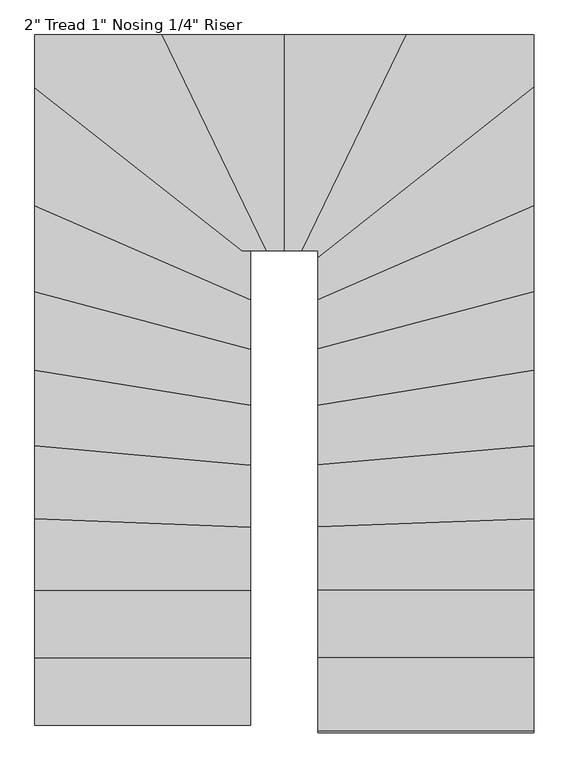
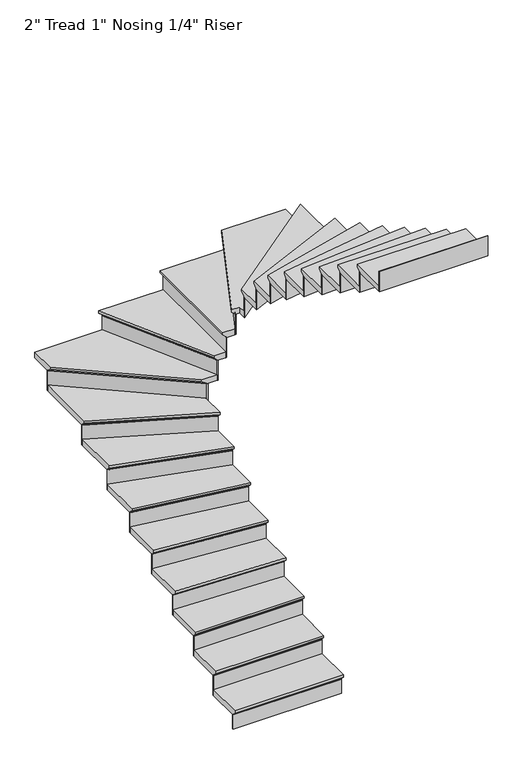
"""IFC4 building model written with IfcOpenShell, lengths in millimetres: stair flight geometry."""

from ifc_helpers import new_model, si_unit, origin, place, context, project, spatial, faceted_brep, source, transform, mapped, element, save


def stair_flight_696a7c4e(model_context):
    return source(origin(), model_context, "Body", "Brep", [
        faceted_brep([(-5047.1987704, -4554.2130548, 7470.3214286), (-5047.1987704, -4554.2130548, 7489.3714286), (-5940.8822214, -4554.2130548, 7489.3714286), (-5940.8822214, -4554.2130548, 7470.3214286), (-5047.1987704, -4528.8130548, 7444.9214286), (-5940.8822214, -4528.8130548, 7444.9214286), (-5047.1987704, -4249.4130548, 7489.3714286), (-5940.8822214, -4249.4130548, 7489.3714286), (-5940.8822214, -4528.8130548, 7438.5714286), (-5940.8822214, -4249.4130548, 7438.5714286), (-5047.1987704, -4249.4130548, 7438.5714286), (-5047.1987704, -4528.8130548, 7438.5714286)], [[[0, 1, 2, 3]], [[4, 0, 3, 5]], [[2, 1, 6, 7]], [[8, 9, 10, 11]], [[2, 7, 9, 8, 5, 3]], [[8, 11, 4, 5]], [[6, 1, 0, 4, 11, 10]], [[7, 6, 10, 9]]]),
        faceted_brep([(-5047.1987704, -4528.8130548, 7438.5714286), (-5047.1987704, -4528.8130548, 7315.2), (-5047.1987704, -4522.4630548, 7315.2), (-5047.1987704, -4522.4630548, 7438.5714286), (-5940.8822214, -4528.8130548, 7438.5714286), (-5940.8822214, -4522.4630548, 7438.5714286), (-5940.8822214, -4522.4630548, 7315.2), (-5940.8822214, -4528.8130548, 7315.2)], [[[0, 1, 2, 3]], [[4, 5, 6, 7]], [[1, 0, 4, 7]], [[2, 1, 7, 6]], [[3, 2, 6, 5]], [[0, 3, 5, 4]]]),
        faceted_brep([(-5047.1987704, -4249.4130548, 7612.7428571), (-5047.1987704, -4249.4130548, 7438.5714286), (-5047.1987704, -4243.0630548, 7438.5714286), (-5047.1987704, -4243.0630548, 7612.7428571), (-5940.8822214, -4249.4130548, 7612.7428571), (-5940.8822214, -4243.0630548, 7612.7428571), (-5940.8822214, -4243.0630548, 7438.5714286), (-5940.8822214, -4249.4130548, 7438.5714286)], [[[0, 1, 2, 3]], [[4, 5, 6, 7]], [[1, 0, 4, 7]], [[2, 1, 7, 6]], [[3, 2, 6, 5]], [[0, 3, 5, 4]]]),
        faceted_brep([(-5940.8822214, -4274.8130548, 7663.5428571), (-5047.1987704, -4274.8130548, 7663.5428571), (-5047.1987704, -3970.0130548, 7663.5428571), (-5940.8822214, -3970.0130548, 7663.5428571), (-5940.8822214, -4249.4130548, 7612.7428571), (-5940.8822214, -3970.0130548, 7612.7428571), (-5047.1987704, -3970.0130548, 7612.7428571), (-5047.1987704, -4249.4130548, 7612.7428571), (-5940.8822214, -4249.4130548, 7619.0928571), (-5940.8822214, -4274.8130548, 7644.4928571), (-5047.1987704, -4249.4130548, 7619.0928571), (-5047.1987704, -4274.8130548, 7644.4928571)], [[[0, 1, 2, 3]], [[4, 5, 6, 7]], [[0, 3, 5, 4, 8, 9]], [[4, 7, 10, 8]], [[2, 1, 11, 10, 7, 6]], [[3, 2, 6, 5]], [[11, 1, 0, 9]], [[10, 11, 9, 8]]]),
        faceted_brep([(-5047.1987704, -3970.0130548, 7786.9142857), (-5047.1987704, -3970.0130548, 7612.7428571), (-5047.1987704, -3963.6630548, 7612.7428571), (-5047.1987704, -3963.6630548, 7786.9142857), (-5940.8822214, -3970.0130548, 7786.9142857), (-5940.8822214, -3963.6630548, 7786.9142857), (-5940.8822214, -3963.6630548, 7612.7428571), (-5940.8822214, -3970.0130548, 7612.7428571)], [[[0, 1, 2, 3]], [[4, 5, 6, 7]], [[1, 0, 4, 7]], [[2, 1, 7, 6]], [[3, 2, 6, 5]], [[0, 3, 5, 4]]]),
        faceted_brep([(-5940.8822214, -3995.4130548, 7837.7142857), (-5047.1987704, -3995.4130548, 7837.7142857), (-5047.1987704, -3707.9036879, 7837.7142857), (-5940.8822214, -3673.2843203, 7837.7142857), (-5940.8822214, -3970.0130548, 7786.9142857), (-5940.8822214, -3673.2843203, 7786.9142857), (-5047.1987704, -3707.9036879, 7786.9142857), (-5047.1987704, -3970.0130548, 7786.9142857), (-5940.8822214, -3970.0130548, 7793.2642857), (-5940.8822214, -3995.4130548, 7818.6642857), (-5047.1987704, -3970.0130548, 7793.2642857), (-5047.1987704, -3995.4130548, 7818.6642857)], [[[0, 1, 2, 3]], [[4, 5, 6, 7]], [[0, 3, 5, 4, 8, 9]], [[4, 7, 10, 8]], [[2, 1, 11, 10, 7, 6]], [[3, 2, 6, 5]], [[11, 1, 0, 9]], [[10, 11, 9, 8]]]),
        faceted_brep([(-5047.1987704, -3707.9036879, 7961.0857143), (-5047.1987704, -3707.9036879, 7786.9142857), (-5047.1987704, -3701.5489252, 7786.9142857), (-5047.1987704, -3701.5489252, 7961.0857143), (-5940.8822214, -3673.2843203, 7961.0857143), (-5940.8822214, -3666.9295576, 7961.0857143), (-5940.8822214, -3666.9295576, 7786.9142857), (-5940.8822214, -3673.2843203, 7786.9142857)], [[[0, 1, 2, 3]], [[4, 5, 6, 7]], [[1, 0, 4, 7]], [[2, 1, 7, 6]], [[3, 2, 6, 5]], [[0, 3, 5, 4]]]),
        faceted_brep([(-5940.8822214, -3698.703371, 8011.8857143), (-5047.1987704, -3733.3227386, 8011.8857143), (-5047.1987704, -3451.3234819, 8011.8857143), (-5940.8822214, -3370.89733, 8011.8857143), (-5940.8822214, -3673.2843203, 7961.0857143), (-5940.8822214, -3370.89733, 7961.0857143), (-5047.1987704, -3451.3234819, 7961.0857143), (-5047.1987704, -3707.9036879, 7961.0857143), (-5940.8822214, -3673.2843203, 7967.4357143), (-5940.8822214, -3698.703371, 7992.8357143), (-5047.1987704, -3707.9036879, 7967.4357143), (-5047.1987704, -3733.3227386, 7992.8357143)], [[[0, 1, 2, 3]], [[4, 5, 6, 7]], [[0, 3, 5, 4, 8, 9]], [[4, 7, 10, 8]], [[2, 1, 11, 10, 7, 6]], [[3, 2, 6, 5]], [[11, 1, 0, 9]], [[10, 11, 9, 8]]]),
        faceted_brep([(-5047.1987704, -3451.3234819, 8135.2571429), (-5047.1987704, -3451.3234819, 7961.0857143), (-5047.1987704, -3444.9478197, 7961.0857143), (-5047.1987704, -3444.9478197, 8135.2571429), (-5940.8822214, -3370.89733, 8135.2571429), (-5940.8822214, -3364.5216678, 8135.2571429), (-5940.8822214, -3364.5216678, 7961.0857143), (-5940.8822214, -3370.89733, 7961.0857143)], [[[0, 1, 2, 3]], [[4, 5, 6, 7]], [[1, 0, 4, 7]], [[2, 1, 7, 6]], [[3, 2, 6, 5]], [[0, 3, 5, 4]]]),
        faceted_brep([(-5940.8822214, -3396.3999789, 8186.0571429), (-5047.1987704, -3476.8261308, 8186.0571429), (-5047.1987704, -3203.4301079, 8186.0571429), (-5940.8822214, -3059.5417727, 8186.0571429), (-5940.8822214, -3370.89733, 8135.2571429), (-5940.8822214, -3059.5417727, 8135.2571429), (-5047.1987704, -3203.4301079, 8135.2571429), (-5047.1987704, -3451.3234819, 8135.2571429), (-5940.8822214, -3370.89733, 8141.6071429), (-5940.8822214, -3396.3999789, 8167.0071429), (-5047.1987704, -3451.3234819, 8141.6071429), (-5047.1987704, -3476.8261308, 8167.0071429)], [[[0, 1, 2, 3]], [[4, 5, 6, 7]], [[0, 3, 5, 4, 8, 9]], [[4, 7, 10, 8]], [[2, 1, 11, 10, 7, 6]], [[3, 2, 6, 5]], [[11, 1, 0, 9]], [[10, 11, 9, 8]]]),
        faceted_brep([(-5047.1987704, -3203.4301079, 8309.4285714), (-5047.1987704, -3203.4301079, 8135.2571429), (-5047.1987704, -3196.9983292, 8135.2571429), (-5047.1987704, -3196.9983292, 8309.4285714), (-5940.8822214, -3059.5417727, 8309.4285714), (-5940.8822214, -3053.109994, 8309.4285714), (-5940.8822214, -3053.109994, 8135.2571429), (-5940.8822214, -3059.5417727, 8135.2571429)], [[[0, 1, 2, 3]], [[4, 5, 6, 7]], [[1, 0, 4, 7]], [[2, 1, 7, 6]], [[3, 2, 6, 5]], [[0, 3, 5, 4]]]),
        faceted_brep([(-5940.8822214, -3085.2688872, 8360.2285714), (-5047.1987704, -3229.1572224, 8360.2285714), (-5047.1987704, -2970.3553609, 8360.2285714), (-5940.8822214, -2732.7052783, 8360.2285714), (-5940.8822214, -3059.5417727, 8309.4285714), (-5940.8822214, -2732.7052783, 8309.4285714), (-5047.1987704, -2970.3553609, 8309.4285714), (-5047.1987704, -3203.4301079, 8309.4285714), (-5940.8822214, -3059.5417727, 8315.7785714), (-5940.8822214, -3085.2688872, 8341.1785714), (-5047.1987704, -3203.4301079, 8315.7785714), (-5047.1987704, -3229.1572224, 8341.1785714)], [[[0, 1, 2, 3]], [[4, 5, 6, 7]], [[0, 3, 5, 4, 8, 9]], [[4, 7, 10, 8]], [[2, 1, 11, 10, 7, 6]], [[3, 2, 6, 5]], [[11, 1, 0, 9]], [[10, 11, 9, 8]]]),
        faceted_brep([(-5047.1987704, -2970.3553609, 8483.6), (-5047.1987704, -2970.3553609, 8309.4285714), (-5047.1987704, -2963.7846771, 8309.4285714), (-5047.1987704, -2963.7846771, 8483.6), (-5940.8822214, -2732.7052783, 8483.6), (-5940.8822214, -2726.1345945, 8483.6), (-5940.8822214, -2726.1345945, 8309.4285714), (-5940.8822214, -2732.7052783, 8309.4285714)], [[[0, 1, 2, 3]], [[4, 5, 6, 7]], [[1, 0, 4, 7]], [[2, 1, 7, 6]], [[3, 2, 6, 5]], [[0, 3, 5, 4]]]),
        faceted_brep([(-5940.8822214, -2758.9880136, 8534.4), (-5047.1987704, -2996.6380961, 8534.4), (-5047.1987704, -2765.8050203, 8534.4), (-5940.8822214, -2375.5896532, 8534.4), (-5940.8822214, -2732.7052783, 8483.6), (-5940.8822214, -2375.5896532, 8483.6), (-5047.1987704, -2765.8050203, 8483.6), (-5047.1987704, -2970.3553609, 8483.6), (-5940.8822214, -2732.7052783, 8489.95), (-5940.8822214, -2758.9880136, 8515.35), (-5047.1987704, -2970.3553609, 8489.95), (-5047.1987704, -2996.6380961, 8515.35)], [[[0, 1, 2, 3]], [[4, 5, 6, 7]], [[0, 3, 5, 4, 8, 9]], [[4, 7, 10, 8]], [[2, 1, 11, 10, 7, 6]], [[3, 2, 6, 5]], [[11, 1, 0, 9]], [[10, 11, 9, 8]]]),
        faceted_brep([(-5047.1987704, -2765.8050203, 8657.7714286), (-5047.1987704, -2765.8050203, 8483.6), (-5047.1987704, -2758.8760908, 8483.6), (-5047.1987704, -2758.8760908, 8657.7714286), (-5940.8822214, -2375.5896532, 8657.7714286), (-5940.8822214, -2368.6607237, 8657.7714286), (-5940.8822214, -2368.6607237, 8483.6), (-5940.8822214, -2375.5896532, 8483.6)], [[[0, 1, 2, 3]], [[4, 5, 6, 7]], [[1, 0, 4, 7]], [[2, 1, 7, 6]], [[3, 2, 6, 5]], [[0, 3, 5, 4]]]),
        faceted_brep([(-5940.8822214, -2403.3053713, 8708.5714286), (-5047.1987704, -2793.5207384, 8708.5714286), (-5047.1987704, -2590.8424524, 8708.5714286), (-5040.8038639, -2590.8424524, 8708.5714286), (-5940.8822214, -1882.1944717, 8708.5714286), (-5940.8822214, -2375.5896532, 8657.7714286), (-5940.8822214, -1882.1944717, 8657.7714286), (-5040.8038639, -2590.8424524, 8657.7714286), (-5047.1987704, -2590.8424524, 8657.7714286), (-5047.1987704, -2765.8050203, 8657.7714286), (-5940.8822214, -2375.5896532, 8664.1214286), (-5940.8822214, -2403.3053713, 8689.5214286), (-5047.1987704, -2765.8050203, 8664.1214286), (-5047.1987704, -2793.5207384, 8689.5214286)], [[[0, 1, 2, 3, 4]], [[5, 6, 7, 8, 9]], [[0, 4, 6, 5, 10, 11]], [[5, 9, 12, 10]], [[2, 1, 13, 12, 9, 8]], [[4, 3, 7, 6]], [[13, 1, 0, 11]], [[12, 13, 11, 10]], [[3, 2, 8, 7]]]),
        faceted_brep([(-5040.8038639, -2590.8424524, 8831.9428571), (-5040.8038639, -2590.8424524, 8657.7714286), (-5030.5387554, -2590.8424524, 8657.7714286), (-5030.5387554, -2590.8424524, 8831.9428571), (-5940.8822214, -1882.1944717, 8831.9428571), (-5940.8822214, -1874.1125661, 8831.9428571), (-5940.8822214, -1874.1125661, 8657.7714286), (-5940.8822214, -1882.1944717, 8657.7714286)], [[[0, 1, 2, 3]], [[4, 5, 6, 7]], [[1, 0, 4, 7]], [[2, 1, 7, 6]], [[3, 2, 6, 5]], [[0, 3, 5, 4]]]),
        faceted_brep([(-5384.6489457, -1697.1590014, 8882.7428571), (-5940.8822214, -1697.1590014, 8882.7428571), (-5940.8822214, -1914.5220945, 8882.7428571), (-5081.8642978, -2590.8424524, 8882.7428571), (-4952.3566185, -2590.8424524, 8882.7428571), (-5940.8822214, -1697.1590014, 8831.9428571), (-5384.6489457, -1697.1590014, 8831.9428571), (-4952.3566185, -2590.8424524, 8831.9428571), (-5040.8038639, -2590.8424524, 8831.9428571), (-5940.8822214, -1882.1944717, 8831.9428571), (-5940.8822214, -1882.1944717, 8838.2928571), (-5940.8822214, -1914.5220945, 8863.6928571), (-5040.8038639, -2590.8424524, 8838.2928571), (-5081.8642978, -2590.8424524, 8863.6928571)], [[[0, 1, 2, 3, 4]], [[5, 6, 7, 8, 9]], [[1, 0, 6, 5]], [[2, 1, 5, 9, 10, 11]], [[9, 8, 12, 10]], [[4, 3, 13, 12, 8, 7]], [[0, 4, 7, 6]], [[13, 3, 2, 11]], [[12, 13, 11, 10]]]),
        faceted_brep([(-4952.3566185, -2590.8424524, 9006.1142857), (-4952.3566185, -2590.8424524, 8831.9428571), (-4945.3027294, -2590.8424524, 8831.9428571), (-4945.3027294, -2590.8424524, 9006.1142857), (-5384.6489457, -1697.1590014, 9006.1142857), (-5377.5950566, -1697.1590014, 9006.1142857), (-5377.5950566, -1697.1590014, 8831.9428571), (-5384.6489457, -1697.1590014, 8831.9428571)], [[[0, 1, 2, 3]], [[4, 5, 6, 7]], [[1, 0, 4, 7]], [[2, 1, 7, 6]], [[3, 2, 6, 5]], [[0, 3, 5, 4]]]),
        faceted_brep([(-5412.8645022, -1697.1590014, 9056.9142857), (-4980.5721749, -2590.8424524, 9056.9142857), (-4882.0987704, -2590.8424524, 9056.9142857), (-4882.0987706, -1697.1590014, 9056.9142857), (-5384.6489457, -1697.1590014, 9006.1142857), (-4882.0987706, -1697.1590014, 9006.1142857), (-4882.0987704, -2590.8424524, 9006.1142857), (-4952.3566185, -2590.8424524, 9006.1142857), (-5384.6489457, -1697.1590014, 9012.4642857), (-5412.8645022, -1697.1590014, 9037.8642857), (-4952.3566185, -2590.8424524, 9012.4642857), (-4980.5721749, -2590.8424524, 9037.8642857)], [[[0, 1, 2, 3]], [[4, 5, 6, 7]], [[0, 3, 5, 4, 8, 9]], [[4, 7, 10, 8]], [[3, 2, 6, 5]], [[11, 1, 0, 9]], [[10, 11, 9, 8]], [[2, 1, 11, 10, 7, 6]]]),
        faceted_brep([(-4882.0987704, -2590.8424524, 9180.2857143), (-4882.0987704, -2590.8424524, 9006.1142857), (-4875.7487704, -2590.8424524, 9006.1142857), (-4875.7487704, -2590.8424524, 9180.2857143), (-4882.0987706, -1697.1590014, 9180.2857143), (-4875.7487706, -1697.1590014, 9180.2857143), (-4875.7487706, -1697.1590014, 9006.1142857), (-4882.0987706, -1697.1590014, 9006.1142857)], [[[0, 1, 2, 3]], [[4, 5, 6, 7]], [[1, 0, 4, 7]], [[2, 1, 7, 6]], [[3, 2, 6, 5]], [[0, 3, 5, 4]]]),
        faceted_brep([(-4907.4987706, -1697.1590014, 9231.0857143), (-4907.4987704, -2590.8424524, 9231.0857143), (-4806.2098095, -2590.8424524, 9231.0857143), (-4373.9174828, -1697.1590014, 9231.0857143), (-4882.0987706, -1697.1590014, 9180.2857143), (-4373.9174828, -1697.1590014, 9180.2857143), (-4806.2098095, -2590.8424524, 9180.2857143), (-4882.0987704, -2590.8424524, 9180.2857143), (-4882.0987706, -1697.1590014, 9186.6357143), (-4907.4987706, -1697.1590014, 9212.0357143), (-4882.0987704, -2590.8424524, 9186.6357143), (-4907.4987704, -2590.8424524, 9212.0357143)], [[[0, 1, 2, 3]], [[4, 5, 6, 7]], [[0, 3, 5, 4, 8, 9]], [[4, 7, 10, 8]], [[2, 1, 11, 10, 7, 6]], [[3, 2, 6, 5]], [[11, 1, 0, 9]], [[10, 11, 9, 8]]]),
        faceted_brep([(-4806.2098095, -2590.8424524, 9354.4571429), (-4806.2098095, -2590.8424524, 9180.2857143), (-4799.1559204, -2590.8424524, 9180.2857143), (-4799.1559204, -2590.8424524, 9354.4571429), (-4373.9174828, -1697.1590014, 9354.4571429), (-4366.8635937, -1697.1590014, 9354.4571429), (-4366.8635937, -1697.1590014, 9180.2857143), (-4373.9174828, -1697.1590014, 9180.2857143)], [[[0, 1, 2, 3]], [[4, 5, 6, 7]], [[1, 0, 4, 7]], [[2, 1, 7, 6]], [[3, 2, 6, 5]], [[0, 3, 5, 4]]]),
        faceted_brep([(-3874.1153195, -1946.8497166, 9405.2571429), (-3874.1153195, -1697.1590014, 9405.2571429), (-4402.1330392, -1697.1590014, 9405.2571429), (-4834.4253659, -2590.8424524, 9405.2571429), (-4767.7987704, -2590.8424524, 9405.2571429), (-4767.7987704, -2650.4628721, 9405.2571429), (-3874.1153195, -1697.1590014, 9354.4571429), (-3874.1153195, -1946.8497166, 9354.4571429), (-4767.7987704, -2650.4628721, 9354.4571429), (-4767.7987704, -2590.8424524, 9354.4571429), (-4806.2098095, -2590.8424524, 9354.4571429), (-4373.9174828, -1697.1590014, 9354.4571429), (-4806.2098095, -2590.8424524, 9360.8071429), (-4373.9174828, -1697.1590014, 9360.8071429), (-4834.4253659, -2590.8424524, 9386.2071429), (-4402.1330392, -1697.1590014, 9386.2071429)], [[[0, 1, 2, 3, 4, 5]], [[6, 7, 8, 9, 10, 11]], [[1, 0, 7, 6]], [[11, 10, 12, 13]], [[4, 3, 14, 12, 10, 9]], [[5, 4, 9, 8]], [[0, 5, 8, 7]], [[14, 3, 2, 15]], [[12, 14, 15, 13]], [[2, 1, 6, 11, 13, 15]]]),
        faceted_brep([(-4767.7987704, -2650.4628721, 9528.6285714), (-4767.7987704, -2650.4628721, 9354.4571429), (-4767.7987704, -2658.5447778, 9354.4571429), (-4767.7987704, -2658.5447778, 9528.6285714), (-3874.1153195, -1946.8497166, 9528.6285714), (-3874.1153195, -1954.9316222, 9528.6285714), (-3874.1153195, -1954.9316222, 9354.4571429), (-3874.1153195, -1946.8497166, 9354.4571429)], [[[0, 1, 2, 3]], [[4, 5, 6, 7]], [[1, 0, 4, 7]], [[2, 1, 7, 6]], [[3, 2, 6, 5]], [[0, 3, 5, 4]]]),
        faceted_brep([(-3874.1153195, -1914.5220938, 9579.4285714), (-4767.7987704, -2618.1352494, 9579.4285714), (-4767.7987704, -2821.2364563, 9579.4285714), (-3874.1153195, -2431.0210889, 9579.4285714), (-3874.1153195, -1946.8497166, 9528.6285714), (-3874.1153195, -2431.0210889, 9528.6285714), (-4767.7987704, -2821.2364563, 9528.6285714), (-4767.7987704, -2650.4628721, 9528.6285714), (-3874.1153195, -1946.8497166, 9534.9785714), (-3874.1153195, -1914.5220938, 9560.3785714), (-4767.7987704, -2650.4628721, 9534.9785714), (-4767.7987704, -2618.1352494, 9560.3785714)], [[[0, 1, 2, 3]], [[4, 5, 6, 7]], [[0, 3, 5, 4, 8, 9]], [[4, 7, 10, 8]], [[2, 1, 11, 10, 7, 6]], [[3, 2, 6, 5]], [[11, 1, 0, 9]], [[10, 11, 9, 8]]]),
        faceted_brep([(-4767.7987704, -2821.2364563, 9702.8), (-4767.7987704, -2821.2364563, 9528.6285714), (-4767.7987704, -2828.1653858, 9528.6285714), (-4767.7987704, -2828.1653858, 9702.8), (-3874.1153195, -2431.0210889, 9702.8), (-3874.1153195, -2437.9500185, 9702.8), (-3874.1153195, -2437.9500185, 9528.6285714), (-3874.1153195, -2431.0210889, 9528.6285714)], [[[0, 1, 2, 3]], [[4, 5, 6, 7]], [[1, 0, 4, 7]], [[2, 1, 7, 6]], [[3, 2, 6, 5]], [[0, 3, 5, 4]]]),
        faceted_brep([(-3874.1153195, -2403.3053709, 9753.6), (-4767.7987704, -2793.5207382, 9753.6), (-4767.7987704, -3022.9208311, 9753.6), (-3874.1153195, -2785.2707484, 9753.6), (-3874.1153195, -2431.0210889, 9702.8), (-3874.1153195, -2785.2707484, 9702.8), (-4767.7987704, -3022.9208311, 9702.8), (-4767.7987704, -2821.2364563, 9702.8), (-3874.1153195, -2431.0210889, 9709.15), (-3874.1153195, -2403.3053709, 9734.55), (-4767.7987704, -2821.2364563, 9709.15), (-4767.7987704, -2793.5207382, 9734.55)], [[[0, 1, 2, 3]], [[4, 5, 6, 7]], [[0, 3, 5, 4, 8, 9]], [[4, 7, 10, 8]], [[2, 1, 11, 10, 7, 6]], [[3, 2, 6, 5]], [[11, 1, 0, 9]], [[10, 11, 9, 8]]]),
        faceted_brep([(-4767.7987704, -3022.9208311, 9876.9714286), (-4767.7987704, -3022.9208311, 9702.8), (-4767.7987704, -3029.4915149, 9702.8), (-4767.7987704, -3029.4915149, 9876.9714286), (-3874.1153195, -2785.2707484, 9876.9714286), (-3874.1153195, -2791.8414322, 9876.9714286), (-3874.1153195, -2791.8414322, 9702.8), (-3874.1153195, -2785.2707484, 9702.8)], [[[0, 1, 2, 3]], [[4, 5, 6, 7]], [[1, 0, 4, 7]], [[2, 1, 7, 6]], [[3, 2, 6, 5]], [[0, 3, 5, 4]]]),
        faceted_brep([(-3874.1153195, -2758.9880132, 9927.7714286), (-4767.7987704, -2996.6380959, 9927.7714286), (-4767.7987704, -3254.8843368, 9927.7714286), (-3874.1153195, -3110.9960015, 9927.7714286), (-3874.1153195, -2785.2707484, 9876.9714286), (-3874.1153195, -3110.9960015, 9876.9714286), (-4767.7987704, -3254.8843368, 9876.9714286), (-4767.7987704, -3022.9208311, 9876.9714286), (-3874.1153195, -2785.2707484, 9883.3214286), (-3874.1153195, -2758.9880132, 9908.7214286), (-4767.7987704, -3022.9208311, 9883.3214286), (-4767.7987704, -2996.6380959, 9908.7214286)], [[[0, 1, 2, 3]], [[4, 5, 6, 7]], [[0, 3, 5, 4, 8, 9]], [[4, 7, 10, 8]], [[2, 1, 11, 10, 7, 6]], [[3, 2, 6, 5]], [[11, 1, 0, 9]], [[10, 11, 9, 8]]]),
        faceted_brep([(-4767.7987704, -3254.8843368, 10051.1428571), (-4767.7987704, -3254.8843368, 9876.9714286), (-4767.7987704, -3261.3161154, 9876.9714286), (-4767.7987704, -3261.3161154, 10051.1428571), (-3874.1153195, -3110.9960015, 10051.1428571), (-3874.1153195, -3117.4277801, 10051.1428571), (-3874.1153195, -3117.4277801, 9876.9714286), (-3874.1153195, -3110.9960015, 9876.9714286)], [[[0, 1, 2, 3]], [[4, 5, 6, 7]], [[1, 0, 4, 7]], [[2, 1, 7, 6]], [[3, 2, 6, 5]], [[0, 3, 5, 4]]]),
        faceted_brep([(-3874.1153195, -3085.2688869, 10101.9428571), (-4767.7987704, -3229.1572222, 10101.9428571), (-4767.7987704, -3502.3287795, 10101.9428571), (-3874.1153195, -3421.9026274, 10101.9428571), (-3874.1153195, -3110.9960015, 10051.1428571), (-3874.1153195, -3421.9026274, 10051.1428571), (-4767.7987704, -3502.3287795, 10051.1428571), (-4767.7987704, -3254.8843368, 10051.1428571), (-3874.1153195, -3110.9960015, 10057.4928571), (-3874.1153195, -3085.2688869, 10082.8928571), (-4767.7987704, -3254.8843368, 10057.4928571), (-4767.7987704, -3229.1572222, 10082.8928571)], [[[0, 1, 2, 3]], [[4, 5, 6, 7]], [[0, 3, 5, 4, 8, 9]], [[4, 7, 10, 8]], [[2, 1, 11, 10, 7, 6]], [[3, 2, 6, 5]], [[11, 1, 0, 9]], [[10, 11, 9, 8]]]),
        faceted_brep([(-4767.7987704, -3502.3287795, 10225.3142857), (-4767.7987704, -3502.3287795, 10051.1428571), (-4767.7987704, -3508.7044417, 10051.1428571), (-4767.7987704, -3508.7044417, 10225.3142857), (-3874.1153195, -3421.9026274, 10225.3142857), (-3874.1153195, -3428.2782897, 10225.3142857), (-3874.1153195, -3428.2782897, 10051.1428571), (-3874.1153195, -3421.9026274, 10051.1428571)], [[[0, 1, 2, 3]], [[4, 5, 6, 7]], [[1, 0, 4, 7]], [[2, 1, 7, 6]], [[3, 2, 6, 5]], [[0, 3, 5, 4]]]),
        faceted_brep([(-3874.1153195, -3396.3999786, 10276.1142857), (-4767.7987704, -3476.8261306, 10276.1142857), (-4767.7987704, -3758.7417891, 10276.1142857), (-3874.1153195, -3724.1224215, 10276.1142857), (-3874.1153195, -3421.9026274, 10225.3142857), (-3874.1153195, -3724.1224215, 10225.3142857), (-4767.7987704, -3758.7417891, 10225.3142857), (-4767.7987704, -3502.3287795, 10225.3142857), (-3874.1153195, -3421.9026274, 10231.6642857), (-3874.1153195, -3396.3999786, 10257.0642857), (-4767.7987704, -3502.3287795, 10231.6642857), (-4767.7987704, -3476.8261306, 10257.0642857)], [[[0, 1, 2, 3]], [[4, 5, 6, 7]], [[0, 3, 5, 4, 8, 9]], [[4, 7, 10, 8]], [[2, 1, 11, 10, 7, 6]], [[3, 2, 6, 5]], [[11, 1, 0, 9]], [[10, 11, 9, 8]]]),
        faceted_brep([(-4767.7987704, -3758.7417891, 10399.4857143), (-4767.7987704, -3758.7417891, 10225.3142857), (-4767.7987704, -3765.0965518, 10225.3142857), (-4767.7987704, -3765.0965518, 10399.4857143), (-3874.1153195, -3724.1224215, 10399.4857143), (-3874.1153195, -3730.4771842, 10399.4857143), (-3874.1153195, -3730.4771842, 10225.3142857), (-3874.1153195, -3724.1224215, 10225.3142857)], [[[0, 1, 2, 3]], [[4, 5, 6, 7]], [[1, 0, 4, 7]], [[2, 1, 7, 6]], [[3, 2, 6, 5]], [[0, 3, 5, 4]]]),
        faceted_brep([(-3874.1153195, -3698.7033708, 10450.2857143), (-4767.7987704, -3733.3227384, 10450.2857143), (-4767.7987704, -4020.8130546, 10450.2857143), (-3874.1153195, -4020.8130546, 10450.2857143), (-3874.1153195, -3724.1224215, 10399.4857143), (-3874.1153195, -4020.8130546, 10399.4857143), (-4767.7987704, -4020.8130546, 10399.4857143), (-4767.7987704, -3758.7417891, 10399.4857143), (-3874.1153195, -3724.1224215, 10405.8357143), (-3874.1153195, -3698.7033708, 10431.2357143), (-4767.7987704, -3758.7417891, 10405.8357143), (-4767.7987704, -3733.3227384, 10431.2357143)], [[[0, 1, 2, 3]], [[4, 5, 6, 7]], [[0, 3, 5, 4, 8, 9]], [[4, 7, 10, 8]], [[2, 1, 11, 10, 7, 6]], [[3, 2, 6, 5]], [[11, 1, 0, 9]], [[10, 11, 9, 8]]]),
        faceted_brep([(-4767.7987704, -4020.8130546, 10573.6571429), (-4767.7987704, -4020.8130546, 10399.4857143), (-4767.7987704, -4027.1630546, 10399.4857143), (-4767.7987704, -4027.1630546, 10573.6571429), (-3874.1153195, -4020.8130546, 10573.6571429), (-3874.1153195, -4027.1630546, 10573.6571429), (-3874.1153195, -4027.1630546, 10399.4857143), (-3874.1153195, -4020.8130546, 10399.4857143)], [[[0, 1, 2, 3]], [[4, 5, 6, 7]], [[1, 0, 4, 7]], [[2, 1, 7, 6]], [[3, 2, 6, 5]], [[0, 3, 5, 4]]]),
        faceted_brep([(-3874.1153195, -3995.4130546, 10624.4571429), (-4767.7987704, -3995.4130546, 10624.4571429), (-4767.7987704, -4300.2130546, 10624.4571429), (-3874.1153195, -4300.2130546, 10624.4571429), (-3874.1153195, -4020.8130546, 10573.6571429), (-3874.1153195, -4300.2130546, 10573.6571429), (-4767.7987704, -4300.2130546, 10573.6571429), (-4767.7987704, -4020.8130546, 10573.6571429), (-3874.1153195, -4020.8130546, 10580.0071429), (-3874.1153195, -3995.4130546, 10605.4071429), (-4767.7987704, -4020.8130546, 10580.0071429), (-4767.7987704, -3995.4130546, 10605.4071429)], [[[0, 1, 2, 3]], [[4, 5, 6, 7]], [[0, 3, 5, 4, 8, 9]], [[4, 7, 10, 8]], [[2, 1, 11, 10, 7, 6]], [[3, 2, 6, 5]], [[11, 1, 0, 9]], [[10, 11, 9, 8]]]),
        faceted_brep([(-4767.7987704, -4300.2130546, 10747.8285714), (-4767.7987704, -4300.2130546, 10573.6571429), (-4767.7987704, -4306.5630546, 10573.6571429), (-4767.7987704, -4306.5630546, 10747.8285714), (-3874.1153195, -4300.2130546, 10747.8285714), (-3874.1153195, -4306.5630546, 10747.8285714), (-3874.1153195, -4306.5630546, 10573.6571429), (-3874.1153195, -4300.2130546, 10573.6571429)], [[[0, 1, 2, 3]], [[4, 5, 6, 7]], [[1, 0, 4, 7]], [[2, 1, 7, 6]], [[3, 2, 6, 5]], [[0, 3, 5, 4]]]),
        faceted_brep([(-4767.7987704, -4579.6130546, 10922.0), (-4767.7987704, -4579.6130546, 10747.8285714), (-4767.7987704, -4585.9630546, 10747.8285714), (-4767.7987704, -4585.9630546, 10922.0), (-3874.1153195, -4579.6130546, 10922.0), (-3874.1153195, -4585.9630546, 10922.0), (-3874.1153195, -4585.9630546, 10747.8285714), (-3874.1153195, -4579.6130546, 10747.8285714)], [[[0, 1, 2, 3]], [[4, 5, 6, 7]], [[1, 0, 4, 7]], [[2, 1, 7, 6]], [[3, 2, 6, 5]], [[0, 3, 5, 4]]]),
        faceted_brep([(-3874.1153195, -4274.8130546, 10798.6285714), (-4767.7987704, -4274.8130546, 10798.6285714), (-4767.7987704, -4579.6130546, 10798.6285714), (-3874.1153195, -4579.6130546, 10798.6285714), (-3874.1153195, -4300.2130546, 10747.8285714), (-3874.1153195, -4579.6130546, 10747.8285714), (-4767.7987704, -4579.6130546, 10747.8285714), (-4767.7987704, -4300.2130546, 10747.8285714), (-3874.1153195, -4300.2130546, 10754.1785714), (-3874.1153195, -4274.8130546, 10779.5785714), (-4767.7987704, -4300.2130546, 10754.1785714), (-4767.7987704, -4274.8130546, 10779.5785714)], [[[0, 1, 2, 3]], [[4, 5, 6, 7]], [[0, 3, 5, 4, 8, 9]], [[4, 7, 10, 8]], [[2, 1, 11, 10, 7, 6]], [[3, 2, 6, 5]], [[11, 1, 0, 9]], [[10, 11, 9, 8]]]),
    ])


if __name__ == "__main__":
    model = new_model("IFC4")
    model_context = context("Model", 3, world=origin())
    ifc_project = project(units=[si_unit("LENGTHUNIT", "METRE", prefix="MILLI")], contexts=[model_context])
    site = spatial("IfcSite", under=ifc_project)
    building = spatial("IfcBuilding", under=site)
    placement = place(None, origin())
    stair_flight_shape = stair_flight_696a7c4e(model_context)
    element("IfcStairFlight", 1, ObjectType="2\" Tread 1\" Nosing 1/4\" Riser", at=placement, inside=building, context=model_context, shape_type="MappedRepresentation", body=[
        mapped(stair_flight_shape, transform((0.0, 0.0, 0.0), x_axis=(1.0, 0.0, 0.0), y_axis=(0.0, 1.0, 0.0), z_axis=(0.0, 0.0, 1.0))),
    ])
    save(model, "model.ifc")

# Revit data of these elements
# Element 1 (IfcStairFlight, "2\" Tread 1\" Nosing 1/4\" Riser")
#   Materials on its faces: "Tile, Porcelain, 4in"
# Materials
#   "Tile, Porcelain, 4in": class "Generic", colour RGB 89 87 158, transparency 0, Description = "Porcelain tile, 4\", white", Cost = 0
